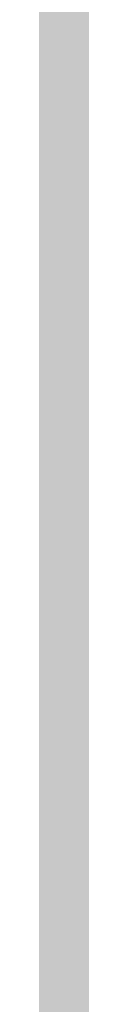
# Model space of a CAD drawing. Units: inches. Extents: x 2083 to 3317, y 1141 to 2115.
# Tile 190 of 256: x 3126.9467 to 3126.9559, y 1263.3548 to 1263.6134. Entities that reach past the tile are written whole.
import ezdxf

# ---------------------------------------------------------------- set-up
doc = ezdxf.new("R2010")
doc.units = ezdxf.units.IN
doc.layers.add('A-ANNO-DIMS', color=2, linetype='Continuous', lineweight=18)
doc.layers.add('A-WALL-PATT', color=251, linetype='Continuous', lineweight=13, true_color=0x636466)
doc.styles.get("Standard").update_dxf_attribs({"font": 'arial.ttf'})
doc.dimstyles.new('ISO-25', dxfattribs={"dimtxt": 12, "dimasz": 12, "dimexe": 1.25, "dimexo": 0.625, "dimtad": 1, "dimlunit": 3, "dimtxsty": 'Standard', "dimcen": 2.5, "dimadec": 0, "dimazin": 0, "dimtfac": 1, "dimtmove": 0, "dimatfit": 3, "dimfxl": 1, "dimarcsym": 0})

# ---------------------------------------------------------------- blocks, each defined once
blk = doc.blocks.new('*D26')
at = {"layer": 'A-ANNO-DIMS', "color": 0, "lineweight": -2, "transparency": 16777216}
for p, q in [((3088.98584, 1274.91509), (3088.98584, 1270.95196)), ((3111.24004, 1274.91509), (3111.24004, 1270.95196)), ((3076.98584, 1272.20196), (2840.26245, 1272.20196)), ((3111.24004, 1272.20196), (3088.98584, 1272.20196)), ((3123.24004, 1272.20196), (3135.24004, 1272.20196))]:
    blk.add_line(p, q, dxfattribs=at)
at = {"layer": 'A-ANNO-DIMS', "color": 0, "transparency": 16777216}
for points in [[(3076.98584, 1274.20196), (3076.98584, 1270.20196), (3088.98584, 1272.20196)], [(3123.24004, 1274.20196), (3123.24004, 1270.20196), (3111.24004, 1272.20196)]]:
    blk.add_solid(points, dxfattribs=at)
at = {"layer": 'Defpoints', "color": 0, "transparency": 16777216}
for p in [(3088.98584, 1275.54009), (3111.24004, 1275.54009), (3088.98584, 1272.20196)]:
    blk.add_point(p, dxfattribs=at)
at = {"layer": 'A-ANNO-DIMS', "color": 0, "transparency": 16777216, "insert": (2952.62415, 1279.0316), "char_height": 12, "attachment_point": 5}
blk.add_mtext('NIGHTSTAND 1\'-10 1/2" TYP.', dxfattribs=at)
blk = doc.blocks.new('*D27')
at = {"layer": 'A-ANNO-DIMS', "color": 0, "lineweight": -2, "transparency": 16777216}
for p, q in [((3114.57817, 1309.79428), (3114.57817, 1321.79428)), ((3111.86504, 1297.79428), (3115.82817, 1297.79428)), ((3114.57817, 1297.79428), (3114.57817, 1275.54009)), ((3111.86504, 1275.54009), (3115.82817, 1275.54009)), ((3114.57817, 1263.54009), (3114.57817, 1140.98859))]:
    blk.add_line(p, q, dxfattribs=at)
at = {"layer": 'A-ANNO-DIMS', "color": 0, "transparency": 16777216}
for points in [[(3112.57817, 1309.79428), (3116.57817, 1309.79428), (3114.57817, 1297.79428)], [(3112.57817, 1263.54009), (3116.57817, 1263.54009), (3114.57817, 1275.54009)]]:
    blk.add_solid(points, dxfattribs=at)
at = {"layer": 'Defpoints', "color": 0, "transparency": 16777216}
for p in [(3111.24004, 1297.79428), (3111.24004, 1275.54009), (3114.57817, 1275.54009)]:
    blk.add_point(p, dxfattribs=at)
at = {"layer": 'A-ANNO-DIMS', "color": 0, "transparency": 16777216, "insert": (3107.74853, 1196.26434), "char_height": 12, "attachment_point": 5, "rotation": 90}
blk.add_mtext('1\'-10 1/2" TYP.', dxfattribs=at)

msp = doc.modelspace()

# ---------------------------------------------------------------- hatches: boundary and pattern name
at = {"layer": 'A-WALL-PATT'}
h = msp.add_hatch(color=256, dxfattribs=at)
h.dxf.hatch_style = 1
h.paths.add_polyline_path([(3126.95978, 2020.76136), (2748.95978, 2020.76136), (2604.95978, 2020.76136), (2226.95978, 2020.76136), (2226.95978, 1702.76136), (2466.95978, 1702.76136), (2466.95978, 1582.76136), (2418.95978, 1582.76136), (2418.95978, 1477.76136), (2226.95978, 1477.76136), (2226.95978, 1263.26136), (2544.95978, 1263.26136), (2544.95978, 1411.76136), (2604.95978, 1411.76136), (2685.95978, 1411.76136), (2685.95978, 1420.76136), (2604.95978, 1420.76136), (2604.95978, 1573.76136), (2604.95978, 1702.76136), (2604.95978, 2011.76136), (2748.95978, 2011.76136), (2748.95978, 1702.76136), (2862.95978, 1702.76136), (2862.95978, 1621.76136), (2871.95978, 1621.76136), (2871.95978, 1702.76136), (2883.95978, 1702.76136), (2883.95978, 1706.93946, -0.026459), (2883.95978, 1711.76136), (2757.95978, 1711.76136), (2757.95978, 1807.76136), (2787.95978, 1807.76136), (2787.95978, 1812.26136), (2757.95978, 1812.26136), (2757.95978, 2011.76136), (2877.95978, 2011.76136), (2877.95978, 1812.26136), (2847.95978, 1812.26136), (2847.95978, 1807.76136), (2889.83574, 1807.76136), (2889.83574, 1812.26136), (2882.45978, 1812.26136), (2882.45978, 2011.76136), (3117.95978, 2011.76136), (3117.95978, 1812.26136), (2937.83574, 1812.26136), (2937.83574, 1807.76136), (2995.70978, 1807.76136), (2995.70978, 1796.11767), (3000.20978, 1796.11767), (3000.20978, 1807.76136), (3117.95978, 1807.76136), (3117.95978, 1711.76136), (3000.20978, 1711.76136), (3000.20978, 1760.11767), (2998.5727, 1760.11767, -0.020711), (2995.70978, 1760.11767), (2995.70978, 1711.76136), (2931.95978, 1711.76136), (2931.95978, 1702.76136), (3126.95978, 1702.76136)])
h.paths.add_polyline_path([(2471.45978, 2011.76136), (2471.45978, 1810.01136), (2462.71694, 1810.01136), (2462.71694, 1805.51136), (2505.95978, 1805.51136), (2505.95978, 1810.01136), (2475.95978, 1810.01136), (2475.95978, 2011.76136), (2595.95978, 2011.76136), (2595.95978, 1810.01136), (2565.95978, 1810.01136), (2565.95978, 1805.51136), (2595.95978, 1805.51136), (2595.95978, 1711.76136), (2235.95978, 1711.76136), (2235.95978, 1805.51136), (2353.70978, 1805.51136), (2353.70978, 1796.05416), (2358.20978, 1796.05416), (2358.20978, 1805.51136), (2414.71694, 1805.51136), (2414.71694, 1810.01136), (2235.95978, 1810.01136), (2235.95978, 2011.76136)], flags=16)
h.paths.add_polyline_path([(2270.20473, 1994.61001), (2270.20473, 1970.61001), (2246.20473, 1970.61001), (2246.20473, 1994.61001)], flags=0)
edge = h.paths.add_edge_path(flags=0)
edge.add_ellipse((2332.02739, 1899.79818), major_axis=(-3.04299, 3.04299), ratio=0.1682525, start_angle=-161.33217, end_angle=-156.30711, ccw=False)
edge.add_ellipse((2333.08204, 1898.74353), major_axis=(-1.05465, 1.05465), ratio=0.4535321, start_angle=-123.37102, end_angle=-94.15911)
edge = h.paths.add_edge_path(flags=0)
edge.add_ellipse((2332.02739, 1968.87629), major_axis=(3.04299, 3.04299), ratio=0.1682525, start_angle=18.66783, end_angle=23.69289)
edge.add_spline(control_points=[(2332.9256, 1970.6911), (2332.22677, 1970.3361), (2330.89371, 1969.65891), (2328.41308, 1970.93214), (2327.20393, 1967.74871), (2324.7096, 1969.95559), (2322.53282, 1967.01235), (2320.01285, 1971.29581), (2317.68031, 1968.15784), (2316.04053, 1967.10205), (2315.4269, 1966.8096)], knot_values=[0, 0, 0, 0, 2.267059, 4.324559, 6.685584, 8.878641, 11.121502, 14.300359, 17.755284, 19.732645, 19.732645, 19.732645, 19.732645], degree=3, periodic=0)
edge.add_ellipse((2332.02739, 1968.87629), major_axis=(3.04299, 3.04299), ratio=0.1682525, start_angle=18.66783, end_angle=23.69289, ccw=False)
edge.add_ellipse((2333.08204, 1969.93094), major_axis=(1.05465, 1.05465), ratio=0.4535321, start_angle=56.62898, end_angle=85.84089, ccw=False)
edge = h.paths.add_edge_path(flags=0)
edge.add_spline(control_points=[(2296.42829, 1967.98791), (2293.6278, 1965.33631), (2287.70362, 1959.72709), (2299.74386, 1949.9957), (2294.53259, 1935.66853), (2290.57323, 1920.60351), (2293.39412, 1909.97369), (2296.18541, 1904.96654)], knot_values=[0.099185, 0.099185, 0.099185, 0.099185, 0.345301, 0.619822, 0.982653, 1.386093, 1.810555, 1.810555, 1.810555, 1.810555], degree=3, periodic=0)
edge.add_spline(control_points=[(2296.18541, 1904.96654), (2297.38358, 1902.6193), (2298.00097, 1901.94931), (2298.55297, 1901.46815)], knot_values=[0.006246, 0.006246, 0.006246, 0.006246, 0.055476, 0.055476, 0.055476, 0.055476], degree=3, periodic=0)
edge.add_spline(control_points=[(2298.55297, 1901.46815), (2297.25861, 1900.92322), (2295.22529, 1900.23213), (2293.06023, 1900.61421), (2292.10142, 1900.78841), (2292.08958, 1900.79057)], knot_values=[0.312835, 0.312835, 0.312835, 0.312835, 0.40178, 0.474987, 0.475903, 0.475903, 0.475903, 0.475903], degree=3, periodic=0)
edge.add_arc((2292.79365, 1904.66411), 3.93701, 215.4209, 259.69818, ccw=False)
edge.add_spline(control_points=[(2289.58531, 1902.3823), (2289.47665, 1902.53509), (2289.36848, 1902.68804), (2289.26086, 1902.84117)], knot_values=[0.102872, 0.102872, 0.102872, 0.102872, 0.116896, 0.116896, 0.116896, 0.116896], degree=3, periodic=0)
edge.add_spline(control_points=[(2289.26086, 1902.84117), (2288.6866, 1902.55019), (2287.64005, 1902.0199), (2285.88134, 1901.87395), (2283.85297, 1901.50435), (2281.71999, 1899.71054), (2278.46699, 1899.49294), (2276.15714, 1901.8832), (2272.25895, 1899.80407), (2267.77761, 1901.84318), (2262.24388, 1900.18403), (2257.41493, 1901.78206), (2254.31837, 1900.72612), (2253.17828, 1900.33734)], knot_values=[0, 0, 0, 0, 1.907977, 3.477176, 5.261074, 7.972851, 11.680248, 13.717921, 16.939592, 22.789562, 27.502503, 33.595215, 37.145618, 37.145618, 37.145618, 37.145618], degree=3, periodic=0)
edge.add_line((2253.17828, 1900.33734), (2250.24424, 1902.84117))
edge.add_line((2250.24424, 1902.84117), (2250.24424, 1965.8333))
edge.add_line((2250.24424, 1965.8333), (2253.17828, 1968.33712))
edge.add_spline(control_points=[(2253.17828, 1968.33712), (2254.31837, 1967.94835), (2257.41493, 1966.89241), (2262.24388, 1968.49043), (2267.77761, 1966.83128), (2271.52673, 1968.53722), (2273.87591, 1967.82829), (2274.2067, 1967.72764)], knot_values=[0, 0, 0, 0, 0.09018, 0.244935, 0.364644, 0.513233, 0.537855, 0.537855, 0.537855, 0.537855], degree=3, periodic=0)
edge.add_arc((2274.35289, 1963.79335), 3.93701, 72.05113, 92.12795, ccw=False)
edge.add_arc((2281.29693, 1985.23), 18.5963, 252.051134, 288.565722)
edge.add_arc((2292.31672, 1956.02888), 12.64608, 71.026788, 113.778218, ccw=False)
edge = h.paths.add_edge_path(flags=0)
edge.add_spline(control_points=[(2274.89941, 1951.85619), (2275.06616, 1951.61659), (2275.23269, 1951.37659), (2275.39799, 1951.13585)], knot_values=[1.409916, 1.409916, 1.409916, 1.409916, 1.43159, 1.43159, 1.43159, 1.43159], degree=3, periodic=0)
edge.add_spline(control_points=[(2275.39799, 1951.13585), (2275.79211, 1950.56189), (2276.17923, 1949.98377), (2276.54555, 1949.3971)], knot_values=[1.358238, 1.358238, 1.358238, 1.358238, 1.409916, 1.409916, 1.409916, 1.409916], degree=3, periodic=0)
edge.add_line((2276.54555, 1949.3971), (2277.43729, 1947.86218))
edge.add_spline(control_points=[(2277.43729, 1947.86218), (2276.30383, 1945.67311), (2274.6397, 1942.42688), (2274.63161, 1938.0939), (2272.79912, 1930.85155), (2274.35643, 1943.89705), (2275.94768, 1947.92336), (2276.54555, 1949.3971)], knot_values=[0.005632, 0.005632, 0.005632, 0.005632, 0.186014, 0.266002, 0.357087, 0.59639, 0.739732, 0.739732, 0.739732, 0.739732], degree=3, periodic=0)
edge.add_spline(control_points=[(2276.54555, 1949.3971), (2276.17923, 1949.98377), (2275.79211, 1950.56189), (2275.39799, 1951.13585)], knot_values=[1.358238, 1.358238, 1.358238, 1.358238, 1.409916, 1.409916, 1.409916, 1.409916], degree=3, periodic=0)
edge.add_spline(control_points=[(2275.39799, 1951.13585), (2274.9425, 1950.08045), (2274.20776, 1948.02527), (2273.9346, 1944.85148), (2272.46853, 1937.62749), (2273.46622, 1945.69647), (2274.70062, 1951.05947), (2274.89941, 1951.85619)], knot_values=[0.104364, 0.104364, 0.104364, 0.104364, 0.189636, 0.269624, 0.36071, 0.600013, 0.644622, 0.644622, 0.644622, 0.644622], degree=3, periodic=0)
h.paths.add_polyline_path([(2269.16751, 1963.12757, -0.357527), (2268.17063, 1960.97637, -0.092561), (2268.17063, 1939.43632, -0.357527), (2269.16751, 1937.28512, -0.357527), (2267.01631, 1938.282, -0.164785), (2254.68558, 1938.282, -0.357527), (2252.53438, 1937.28512, -0.357527), (2253.53126, 1939.43632, -0.092561), (2253.53126, 1960.97637, -0.357527), (2252.53438, 1963.12757, -0.357527), (2254.68558, 1962.13069, -0.164785), (2267.01631, 1962.13069, -0.357527)], flags=0)
h.paths.add_polyline_path([(2248.87407, 1967.8018), (2248.87407, 1957.02771), (2249.45778, 1957.02771), (2249.45778, 1911.64676), (2248.87407, 1911.64676), (2248.87407, 1900.87267), (2246.51186, 1900.87267, 0.197327), (2244.14966, 1902.45687), (2244.14966, 1966.21759, 0.197327), (2246.51186, 1967.8018)], flags=0)
h.paths.add_polyline_path([(2269.16751, 1931.38934, -0.357527), (2268.17063, 1929.23814, -0.092561), (2268.17063, 1907.6981, -0.357527), (2269.16751, 1905.54689, -0.357527), (2267.01631, 1906.54377, -0.164785), (2254.68558, 1906.54377, -0.357527), (2252.53438, 1905.54689, -0.357527), (2253.53126, 1907.6981, -0.092561), (2253.53126, 1929.23814, -0.357527), (2252.53438, 1931.38934, -0.357527), (2254.68558, 1930.39246, -0.164785), (2267.01631, 1930.39246, -0.357527)], flags=0)
edge = h.paths.add_edge_path(flags=0)
edge.add_spline(control_points=[(2276.19686, 1906.7237), (2276.16814, 1909.02893), (2276.11405, 1913.37185), (2270.59842, 1924.92498), (2273.90517, 1919.01278), (2275.92171, 1916.26206), (2275.47457, 1912.40215), (2277.25787, 1910.38062), (2276.69604, 1908.22504), (2276.64622, 1906.81302), (2276.61782, 1906.00841)], knot_values=[0, 0, 0, 0, 8.61026, 16.221274, 18.843057, 23.804898, 27.440828, 29.356102, 31.203478, 33.650687, 33.650687, 33.650687, 33.650687], degree=3, periodic=0)
edge.add_spline(control_points=[(2276.61782, 1906.00841), (2276.62331, 1905.62414), (2276.49774, 1904.62866), (2275.44178, 1903.85473), (2274.93731, 1903.08045), (2274.85908, 1902.84117)], knot_values=[0.156488, 0.156488, 0.156488, 0.156488, 0.184398, 0.231376, 0.250598, 0.250598, 0.250598, 0.250598], degree=3, periodic=0)
edge.add_line((2274.85908, 1902.84117), (2276.50598, 1902.84117))
edge.add_spline(control_points=[(2276.50598, 1902.84117), (2276.78831, 1903.08494), (2277.66507, 1904.1252), (2278.24954, 1904.34074), (2277.65387, 1908.52739), (2278.15567, 1906.22781), (2278.10046, 1905.28595), (2278.84667, 1904.06901), (2277.85679, 1903.41495), (2277.87419, 1902.99105), (2277.90356, 1902.84117)], knot_values=[0.059574, 0.059574, 0.059574, 0.059574, 0.080753, 0.103741, 0.16972, 0.176036, 0.207137, 0.240474, 0.262341, 0.27366, 0.27366, 0.27366, 0.27366], degree=3, periodic=0)
edge.add_line((2277.90356, 1902.84117), (2280.02983, 1902.84117))
edge.add_spline(control_points=[(2280.02983, 1902.84117), (2279.88822, 1903.0884), (2279.49926, 1903.98155), (2280.15228, 1905.93935), (2278.10362, 1909.65776), (2279.76239, 1907.18529), (2280.3279, 1904.87486), (2280.48511, 1903.48959), (2281.46327, 1903.24943), (2281.75834, 1902.9365), (2281.83404, 1902.84117)], knot_values=[0.013856, 0.013856, 0.013856, 0.013856, 0.034874, 0.088867, 0.107879, 0.126738, 0.158714, 0.193757, 0.217487, 0.226722, 0.226722, 0.226722, 0.226722], degree=3, periodic=0)
edge.add_spline(control_points=[(2281.83404, 1902.84117), (2281.78753, 1902.8267), (2281.64702, 1902.78299), (2281.39553, 1902.85949), (2281.08808, 1902.98524), (2280.72068, 1903.0609), (2280.33345, 1903.02573), (2280.12477, 1902.89888), (2280.02983, 1902.84117)], knot_values=[0, 0, 0, 0, 0.14413, 0.435517, 0.749276, 1.153046, 1.548371, 1.878348, 1.878348, 1.878348, 1.878348], degree=3, periodic=0)
edge.add_line((2280.02983, 1902.84117), (2277.90356, 1902.84117))
edge.add_spline(control_points=[(2277.90356, 1902.84117), (2277.89286, 1902.79586), (2277.8654, 1902.67964), (2277.60748, 1902.68748), (2277.27405, 1902.8007), (2276.83792, 1902.61977), (2276.58381, 1902.78926), (2276.50598, 1902.84117)], knot_values=[0, 0, 0, 0, 0.127189, 0.326199, 0.628009, 1.24357, 1.515331, 1.515331, 1.515331, 1.515331], degree=3, periodic=0)
edge.add_line((2276.50598, 1902.84117), (2274.85908, 1902.84117))
edge.add_spline(control_points=[(2274.85908, 1902.84117), (2274.81444, 1902.89859), (2274.72513, 1903.01345), (2274.49348, 1903.11897), (2274.24429, 1902.96054), (2273.93712, 1903.18494), (2273.61404, 1902.98314), (2273.40832, 1902.88304), (2273.32225, 1902.84117)], knot_values=[0, 0, 0, 0, 0.21843, 0.436957, 0.687977, 0.990379, 1.398396, 1.69185, 1.69185, 1.69185, 1.69185], degree=3, periodic=0)
edge.add_spline(control_points=[(2273.32225, 1902.84117), (2273.61674, 1903.44569), (2274.274, 1904.53825), (2276.02724, 1904.5737), (2276.20696, 1906.58364), (2276.19686, 1906.7237)], knot_values=[0.012227, 0.012227, 0.012227, 0.012227, 0.059472, 0.106218, 0.134458, 0.134458, 0.134458, 0.134458], degree=3, periodic=0)
h.paths.add_polyline_path([(2270.77605, 1897.78983), (2270.77605, 1873.78983), (2246.77605, 1873.78983), (2246.77605, 1897.78983)], flags=0)
h.paths.add_polyline_path([(2353.70978, 1760.00506), (2353.70978, 1760.05416), (2358.20978, 1760.05416, -0.033729)], flags=0)
h.paths.add_polyline_path([(2321.81912, 1737.52919), (2341.99533, 1737.52919, -0.414214), (2343.20327, 1736.32124), (2343.20327, 1721.0206, -0.414214), (2341.99533, 1719.81265), (2321.81912, 1719.81265, -0.414214), (2320.61117, 1721.0206), (2320.61117, 1736.32124, -0.414214)], flags=0)
h.paths.add_polyline_path([(2324.23501, 1736.32124), (2339.57944, 1736.32124, -0.414214), (2341.99533, 1733.90535), (2341.99533, 1725.44973, -0.414214), (2339.57944, 1723.03384), (2333.68059, 1723.03384), (2333.84532, 1722.04547, -0.870646), (2335.4254, 1721.82589, -0.767327), (2333.92269, 1721.42324), (2331.29102, 1721.42324, -0.767327), (2329.78832, 1721.82589, -0.870646), (2331.3684, 1722.04547), (2331.53313, 1723.03384), (2324.23501, 1723.03384, -0.414214), (2321.81912, 1725.44973), (2321.81912, 1733.90535, -0.414214)], flags=0)
h.paths.add_polyline_path([(2570.48379, 1928.61544), (2589.68379, 1928.61544), (2590.16883, 1928.61544), (2590.16883, 1904.9934), (2570.48379, 1904.9934)], flags=0)
h.paths.add_polyline_path([(2574.44732, 1927.26382, -1), (2572.82884, 1927.26382, -1)], flags=0)
h.paths.add_polyline_path([(2573.08987, 1926.94088), (2573.92503, 1927.77604), (2574.14774, 1927.55333), (2573.31258, 1926.71817)], flags=0)
h.paths.add_polyline_path([(2578.77906, 1919.72962, -1), (2571.59166, 1919.72962, -1)], flags=0)
h.paths.add_polyline_path([(2578.38536, 1919.72962, -1), (2571.98536, 1919.72962, -1)], flags=0)
h.paths.add_polyline_path([(2331.59576, 1729.47622, -1), (2333.61795, 1729.47622, -1)], flags=0)
h.paths.add_polyline_path([(2578.03423, 1927.26382, -1), (2576.41574, 1927.26382, -1)], flags=0)
h.paths.add_polyline_path([(2576.68885, 1927.53109), (2576.91156, 1927.7538), (2577.74673, 1926.91863), (2577.52402, 1926.69592)], flags=0)
h.paths.add_polyline_path([(2578.13906, 1909.85954, -1), (2572.23166, 1909.85954, -1)], flags=0)
h.paths.add_polyline_path([(2577.74536, 1909.85954, -1), (2572.62536, 1909.85954, -1)], flags=0)
h.paths.add_polyline_path([(2583.79772, 1927.26382, -1), (2582.17923, 1927.26382, -1)], flags=0)
h.paths.add_polyline_path([(2582.71865, 1927.7538), (2583.55381, 1926.91863), (2583.3311, 1926.69592), (2582.49594, 1927.53109)], flags=0)
h.paths.add_polyline_path([(2582.49594, 1927.53109), (2582.71865, 1927.7538), (2583.55381, 1926.91863), (2583.3311, 1926.69592)], flags=0)
h.paths.add_polyline_path([(2587.73906, 1920.52962, -1), (2581.83166, 1920.52962, -1)], flags=0)
h.paths.add_polyline_path([(2587.34536, 1920.52962, -1), (2582.22536, 1920.52962, -1)], flags=0)
h.paths.add_polyline_path([(2587.38462, 1927.26382, -1), (2585.76613, 1927.26382, -1)], flags=0)
h.paths.add_polyline_path([(2586.08199, 1926.98025), (2586.91716, 1927.81541), (2587.13987, 1927.5927), (2586.3047, 1926.75754)], flags=0)
h.paths.add_polyline_path([(2588.37906, 1910.65954, -1), (2581.19166, 1910.65954, -1)], flags=0)
h.paths.add_polyline_path([(2587.98536, 1910.65954, -1), (2581.58536, 1910.65954, -1)], flags=0)
h.paths.add_polyline_path([(2417.16773, 1729.4779), (2437.34394, 1729.4779, -0.414214), (2438.55188, 1728.26995), (2438.55188, 1712.96931, -0.414214), (2437.34394, 1711.76136), (2417.16773, 1711.76136, -0.414214), (2415.95978, 1712.96931), (2415.95978, 1728.26995, -0.414214)], flags=0)
h.paths.add_polyline_path([(2419.58362, 1728.26995), (2434.92805, 1728.26995, -0.414214), (2437.34394, 1725.85406), (2437.34394, 1717.39844, -0.414214), (2434.92805, 1714.98255), (2429.0292, 1714.98255), (2429.19393, 1713.99418, -0.870646), (2430.77401, 1713.7746, -0.767327), (2429.2713, 1713.37195), (2426.63963, 1713.37195, -0.767327), (2425.13693, 1713.7746, -0.870646), (2426.71701, 1713.99418), (2426.88174, 1714.98255), (2419.58362, 1714.98255, -0.414214), (2417.16773, 1717.39844), (2417.16773, 1725.85406, -0.414214)], flags=0)
h.paths.add_polyline_path([(2419.58362, 1728.26995), (2434.92805, 1728.26995, -0.414214), (2437.34394, 1725.85406), (2437.34394, 1717.39844, -0.414214), (2434.92805, 1714.98255), (2429.0292, 1714.98255), (2428.35812, 1719.00903), (2427.55282, 1719.00903), (2426.88174, 1714.98255), (2419.58362, 1714.98255, -0.414214), (2417.16773, 1717.39844), (2417.16773, 1725.85406, -0.414214)], flags=0)
h.paths.add_polyline_path([(2426.94437, 1721.42492, -1), (2428.96656, 1721.42492, -1)], flags=0)
h.paths.add_polyline_path([(2475.95978, 1702.76136), (2595.95978, 1702.76136), (2595.95978, 1582.76136), (2475.95978, 1582.76136)], flags=16)
h.paths.add_polyline_path([(2427.95978, 1573.76136), (2595.95978, 1573.76136), (2595.95978, 1468.76136), (2595.95978, 1420.76136), (2384.45978, 1420.76136), (2384.45978, 1468.76136), (2427.95978, 1468.76136)], flags=16)
h.paths.add_polyline_path([(2379.95978, 1468.76136), (2379.95978, 1420.76136), (2235.95978, 1420.76136), (2235.95978, 1468.76136)], flags=16)
h.paths.add_polyline_path([(2317.816, 1466.69577), (2337.9922, 1466.69577, -0.414214), (2339.20015, 1465.48782), (2339.20015, 1450.18718, -0.414214), (2337.9922, 1448.97923), (2317.816, 1448.97923, -0.414214), (2316.60805, 1450.18718), (2316.60805, 1465.48782, -0.414214)], flags=0)
h.paths.add_polyline_path([(2320.23189, 1465.48782), (2335.57631, 1465.48782, -0.414214), (2337.9922, 1463.07193), (2337.9922, 1454.61631, -0.414214), (2335.57631, 1452.20042), (2329.67747, 1452.20042), (2329.84219, 1451.21205, -0.870646), (2331.42228, 1450.99247, -0.767327), (2329.91957, 1450.58983), (2327.2879, 1450.58983, -0.767327), (2325.7852, 1450.99247, -0.870646), (2327.36528, 1451.21205), (2327.53001, 1452.20042), (2320.23189, 1452.20042, -0.414214), (2317.816, 1454.61631), (2317.816, 1463.07193, -0.414214)], flags=0)
h.paths.add_polyline_path([(2320.23189, 1465.48782), (2335.57631, 1465.48782, -0.414214), (2337.9922, 1463.07193), (2337.9922, 1454.61631, -0.414214), (2335.57631, 1452.20042), (2329.67747, 1452.20042), (2329.00638, 1456.22691), (2328.20109, 1456.22691), (2327.53001, 1452.20042), (2320.23189, 1452.20042, -0.414214), (2317.816, 1454.61631), (2317.816, 1463.07193, -0.414214)], flags=0)
h.paths.add_polyline_path([(2327.59264, 1458.6428, -1), (2329.61483, 1458.6428, -1)], flags=0)
h.paths.add_polyline_path([(2244.41174, 1433.34045), (2241.92094, 1433.34045, -0.414214), (2240.01786, 1435.24354), (2240.01786, 1440.95281, -0.414211), (2241.92093, 1442.8559), (2244.41174, 1442.8559, -1.976472)], flags=0)
h.paths.add_polyline_path([(2245.35689, 1434.39754, -0.414214), (2245.35689, 1441.79881, -2.144098)], flags=0)
h.paths.add_polyline_path([(2535.95978, 1416.26136), (2535.95978, 1272.26136), (2235.95978, 1272.26136), (2235.95978, 1416.26136)], flags=16)
h.paths.add_polyline_path([(2260.11956, 1384.29284), (2260.11956, 1362.03865), (2237.86537, 1362.03865), (2237.86537, 1384.29284)], flags=0)
edge = h.paths.add_edge_path(flags=0)
edge.add_line((2318.25185, 1362.0933), (2318.1458, 1362.00097))
edge.add_ellipse((2317.44512, 1360.43104), major_axis=(2.82164, 2.82164), ratio=0.1682525, start_angle=18.66783, end_angle=20.94813, ccw=False)
edge.add_ellipse((2318.42305, 1361.40897), major_axis=(0.97793, 0.97793), ratio=0.4535321, start_angle=56.62898, end_angle=70.2262, ccw=False)
edge = h.paths.add_edge_path(flags=0)
edge.add_line((2319.10737, 1295.57108), (2319.01504, 1295.67713))
edge.add_ellipse((2317.44512, 1296.37781), major_axis=(-2.82164, 2.82164), ratio=0.1682525, start_angle=-161.33217, end_angle=-159.05187, ccw=False)
edge.add_ellipse((2318.42305, 1295.39988), major_axis=(-0.97793, 0.97793), ratio=0.4535321, start_angle=-123.37102, end_angle=-109.7738)
edge = h.paths.add_edge_path(flags=0)
edge.add_spline(control_points=[(2284.21035, 1301.17022), (2284.58069, 1300.44472), (2284.89119, 1299.89202), (2285.15955, 1299.46102)], knot_values=[0.039066, 0.039066, 0.039066, 0.039066, 0.055476, 0.055476, 0.055476, 0.055476], degree=3, periodic=0)
edge.add_line((2285.15955, 1299.46102), (2284.21035, 1301.17022))
edge = h.paths.add_edge_path(flags=0)
edge.add_line((2280.41246, 1297.29801), (2283.36999, 1297.03612))
edge.add_line((2283.36999, 1297.03612), (2286.40569, 1297.92631))
edge.add_spline(control_points=[(2286.40569, 1297.92631), (2285.30549, 1297.46312), (2284.34478, 1297.12915), (2283.36999, 1297.03612)], knot_values=[0.394369, 0.394369, 0.394369, 0.394369, 0.475903, 0.475903, 0.475903, 0.475903], degree=3, periodic=0)
edge.add_spline(control_points=[(2283.36999, 1297.03612), (2283.28139, 1297.02767), (2282.31629, 1296.95734), (2281.3125, 1297.13448), (2280.42344, 1297.29602), (2280.41246, 1297.29801)], knot_values=[0.312835, 0.312835, 0.312835, 0.312835, 0.320246, 0.393453, 0.394369, 0.394369, 0.394369, 0.394369], degree=3, periodic=0)
edge = h.paths.add_edge_path(flags=0)
edge.add_line((2284.43556, 1359.60729), (2280.44629, 1355.32805))
edge.add_line((2280.44629, 1355.32805), (2279.57999, 1351.01775))
edge.add_line((2279.57999, 1351.01775), (2282.41297, 1346.58043))
edge.add_spline(control_points=[(2282.41297, 1346.58043), (2283.15333, 1345.58924), (2284.2529, 1344.0289), (2284.80104, 1342.38717), (2284.93516, 1341.80554)], knot_values=[1.240098, 1.240098, 1.240098, 1.240098, 1.332892, 1.382712, 1.382712, 1.382712, 1.382712], degree=3, periodic=0)
edge.add_spline(control_points=[(2284.93516, 1341.80554), (2285.31911, 1340.1406), (2285.23303, 1338.4092), (2284.90994, 1336.65412)], knot_values=[1.097484, 1.097484, 1.097484, 1.097484, 1.240098, 1.240098, 1.240098, 1.240098], degree=3, periodic=0)
edge.add_spline(control_points=[(2284.90994, 1336.65412), (2284.58685, 1334.89904), (2284.02675, 1333.12027), (2283.46264, 1331.36058)], knot_values=[0.95487, 0.95487, 0.95487, 0.95487, 1.097484, 1.097484, 1.097484, 1.097484], degree=3, periodic=0)
edge.add_line((2283.46264, 1331.36058), (2281.89038, 1326.15336))
edge.add_line((2281.89038, 1326.15336), (2280.75626, 1321.05609))
edge.add_line((2280.75626, 1321.05609), (2280.2992, 1316.00198))
edge.add_line((2280.2992, 1316.00198), (2280.71593, 1310.95007))
edge.add_line((2280.71593, 1310.95007), (2282.02809, 1305.97214))
edge.add_line((2282.02809, 1305.97214), (2284.21035, 1301.17022))
edge.add_spline(control_points=[(2284.21035, 1301.17022), (2283.34073, 1302.73019), (2282.6119, 1304.33649), (2282.02809, 1305.97214)], knot_values=[0.099185, 0.099185, 0.099185, 0.099185, 0.241799, 0.241799, 0.241799, 0.241799], degree=3, periodic=0)
edge.add_spline(control_points=[(2282.02809, 1305.97214), (2281.44428, 1307.60778), (2281.00549, 1309.27276), (2280.71593, 1310.95007)], knot_values=[0.241799, 0.241799, 0.241799, 0.241799, 0.384413, 0.384413, 0.384413, 0.384413], degree=3, periodic=0)
edge.add_spline(control_points=[(2280.71593, 1310.95007), (2280.43324, 1312.58761), (2280.28939, 1314.27696), (2280.29889, 1315.96203), (2280.2992, 1316.00198)], knot_values=[0.384413, 0.384413, 0.384413, 0.384413, 0.523647, 0.527028, 0.527028, 0.527028, 0.527028], degree=3, periodic=0)
edge.add_spline(control_points=[(2280.2992, 1316.00198), (2280.31233, 1317.68696), (2280.47787, 1319.36793), (2280.75626, 1321.05609)], knot_values=[0.527028, 0.527028, 0.527028, 0.527028, 0.669642, 0.669642, 0.669642, 0.669642], degree=3, periodic=0)
edge.add_spline(control_points=[(2280.75626, 1321.05609), (2281.03465, 1322.74425), (2281.42588, 1324.43961), (2281.89038, 1326.15336)], knot_values=[0.669642, 0.669642, 0.669642, 0.669642, 0.812256, 0.812256, 0.812256, 0.812256], degree=3, periodic=0)
edge.add_spline(control_points=[(2281.89038, 1326.15336), (2282.26438, 1327.53325), (2282.78787, 1329.26181), (2283.35275, 1331.01778), (2283.46264, 1331.36058)], knot_values=[0.812256, 0.812256, 0.812256, 0.812256, 0.927087, 0.95487, 0.95487, 0.95487, 0.95487], degree=3, periodic=0)
edge.add_line((2283.46264, 1331.36058), (2284.90994, 1336.65412))
edge.add_line((2284.90994, 1336.65412), (2284.93516, 1341.80554))
edge.add_line((2284.93516, 1341.80554), (2282.41297, 1346.58043))
edge.add_spline(control_points=[(2282.41297, 1346.58043), (2281.27513, 1348.10379), (2280.07845, 1349.57032), (2279.57999, 1351.01775)], knot_values=[1.382712, 1.382712, 1.382712, 1.382712, 1.525326, 1.525326, 1.525326, 1.525326], degree=3, periodic=0)
edge.add_spline(control_points=[(2279.57999, 1351.01775), (2279.44328, 1351.41472), (2279.13631, 1352.85692), (2279.73519, 1354.29039), (2280.44629, 1355.32805)], knot_values=[1.525326, 1.525326, 1.525326, 1.525326, 1.564439, 1.667941, 1.667941, 1.667941, 1.667941], degree=3, periodic=0)
edge.add_spline(control_points=[(2280.44629, 1355.32805), (2281.42611, 1356.75784), (2282.93084, 1358.18256), (2284.43556, 1359.60729)], knot_values=[1.667941, 1.667941, 1.667941, 1.667941, 1.810555, 1.810555, 1.810555, 1.810555], degree=3, periodic=0)
edge.add_arc((2280.62307, 1348.51818), 11.72618, 71.026788, 113.778218)
edge.add_arc((2270.40489, 1375.59516), 17.24357, 252.051134, 288.565722, ccw=False)
edge.add_arc((2263.96597, 1355.71785), 3.65062, 72.05113, 92.12795)
edge.add_arc((2263.96597, 1355.71785), 3.65062, 92.12795, 177.98513)
edge.add_spline(control_points=[(2260.3176, 1355.8462), (2260.26042, 1354.22067), (2260.55128, 1350.18655), (2262.99934, 1346.76625), (2264.47274, 1344.64902)], knot_values=[1.43159, 1.43159, 1.43159, 1.43159, 1.564144, 1.770695, 1.770695, 1.770695, 1.770695], degree=3, periodic=0)
edge.add_line((2264.47274, 1344.64902), (2264.93559, 1343.98253))
edge.add_spline(control_points=[(2263.80104, 1340.24811), (2263.84324, 1340.51409), (2264.06724, 1341.75647), (2264.51269, 1343.00245), (2264.93505, 1343.98108)], knot_values=[0.53657, 0.53657, 0.53657, 0.53657, 0.559349, 0.644622, 0.644622, 0.644622, 0.644622], degree=3, periodic=0)
edge.add_spline(control_points=[(2264.93505, 1343.98108), (2265.11777, 1343.71497), (2265.29888, 1343.44791), (2265.47676, 1343.17936)], knot_values=[1.384077, 1.384077, 1.384077, 1.384077, 1.409916, 1.409916, 1.409916, 1.409916], degree=3, periodic=0)
edge.add_spline(control_points=[(2265.47676, 1343.17936), (2265.65464, 1342.91082), (2265.8293, 1342.64081), (2265.99913, 1342.36881)], knot_values=[1.358238, 1.358238, 1.358238, 1.358238, 1.384077, 1.384077, 1.384077, 1.384077], degree=3, periodic=0)
edge.add_line((2265.99913, 1342.36881), (2266.82601, 1340.94555))
edge.add_spline(control_points=[(2266.82601, 1340.94555), (2268.8944, 1337.08969), (2271.39817, 1325.843), (2270.51616, 1310.56856), (2275.91938, 1301.86061), (2277.78951, 1299.19945)], knot_values=[0.116896, 0.116896, 0.116896, 0.116896, 0.472987, 1.050969, 1.313793, 1.313793, 1.313793, 1.313793], degree=3, periodic=0)
edge.add_spline(control_points=[(2277.78951, 1299.19945), (2277.83941, 1299.12845), (2277.88943, 1299.0575), (2277.93957, 1298.98658)], knot_values=[0.109884, 0.109884, 0.109884, 0.109884, 0.116896, 0.116896, 0.116896, 0.116896], degree=3, periodic=0)
edge.add_line((2277.93957, 1298.98658), (2277.78885, 1299.19911))
edge.add_spline(control_points=[(2277.78885, 1299.19911), (2277.25658, 1298.92941), (2276.28635, 1298.4379), (2275.03935, 1298.33442), (2274.38333, 1298.2389), (2274.21525, 1298.20934)], knot_values=[33.12187, 33.12187, 33.12187, 33.12187, 35.029056, 36.598255, 37.144827, 37.144827, 37.144827, 37.144827], degree=3, periodic=0)
edge.add_line((2274.21525, 1298.20934), (2273.07315, 1297.89296))
edge.add_spline(control_points=[(2273.07315, 1297.89296), (2272.32294, 1297.57978), (2271.03915, 1296.51051), (2269.24839, 1296.22606), (2268.4231, 1296.37465)], knot_values=[26.532584, 26.532584, 26.532584, 26.532584, 29.198919, 31.839101, 31.839101, 31.839101, 31.839101], degree=3, periodic=0)
edge.add_line((2268.4231, 1296.37465), (2263.8785, 1297.45753))
edge.add_spline(control_points=[(2263.8785, 1297.45753), (2263.55608, 1297.35943), (2261.86031, 1296.83869), (2260.23878, 1297.28241), (2258.93345, 1297.51646)], knot_values=[15.919551, 15.919551, 15.919551, 15.919551, 16.939592, 21.226067, 21.226067, 21.226067, 21.226067], degree=3, periodic=0)
edge.add_line((2258.93345, 1297.51646), (2254.05523, 1297.32901))
edge.add_spline(control_points=[(2254.05523, 1297.32901), (2253.75553, 1297.29582), (2252.11368, 1297.16517), (2250.46187, 1297.54422), (2249.12969, 1297.66788)], knot_values=[5.306517, 5.306517, 5.306517, 5.306517, 6.276435, 10.613034, 10.613034, 10.613034, 10.613034], degree=3, periodic=0)
edge.add_line((2249.12969, 1297.66788), (2244.33165, 1296.87776))
edge.add_line((2244.33165, 1296.87776), (2241.61103, 1299.19945))
edge.add_line((2241.61103, 1299.19945), (2241.61103, 1357.6094))
edge.add_line((2241.61103, 1357.6094), (2244.33165, 1359.9311))
edge.add_line((2244.33165, 1359.9311), (2252.72882, 1359.54269))
edge.add_spline(control_points=[(2252.72882, 1359.54269), (2252.87094, 1359.54644), (2253.30574, 1359.54817), (2253.73984, 1359.51427), (2254.03174, 1359.48243)], knot_values=[0.233291, 0.233291, 0.233291, 0.233291, 0.244935, 0.268927, 0.268927, 0.268927, 0.268927], degree=3, periodic=0)
edge.add_line((2254.03174, 1359.48243), (2259.58719, 1359.41639))
edge.add_spline(control_points=[(2259.58719, 1359.41639), (2260.67707, 1359.6285), (2262.0732, 1359.897), (2263.52369, 1359.45928), (2263.83042, 1359.36595)], knot_values=[0.422516, 0.422516, 0.422516, 0.422516, 0.513233, 0.537855, 0.537855, 0.537855, 0.537855], degree=3, periodic=0)
edge.add_arc((2263.96597, 1355.71785), 3.65062, 72.05113, 92.12795, ccw=False)
edge.add_arc((2270.40489, 1375.59516), 17.24357, 252.051134, 288.565722)
edge.add_arc((2280.62307, 1348.51818), 11.72618, 71.026788, 113.778218, ccw=False)
h.paths.add_polyline_path([(2240.34053, 1359.43471), (2240.34053, 1349.44435), (2240.88178, 1349.44435), (2240.88178, 1307.3645), (2240.34053, 1307.3645), (2240.34053, 1297.37414), (2238.15016, 1297.37414, 0.197327), (2235.95978, 1298.84311), (2235.95978, 1357.96575, 0.197327), (2238.15016, 1359.43471)], flags=0)
h.paths.add_polyline_path([(2259.15779, 1355.1005, -0.357527), (2258.23342, 1353.10578, -0.092561), (2258.23342, 1333.1326, -0.357527), (2259.15779, 1331.13788, -0.357527), (2257.16307, 1332.06225, -0.164785), (2245.7293, 1332.06225, -0.357527), (2243.73458, 1331.13788, -0.357527), (2244.65895, 1333.1326, -0.092561), (2244.65895, 1353.10578, -0.357527), (2243.73458, 1355.1005, -0.357527), (2245.7293, 1354.17613, -0.164785), (2257.16307, 1354.17613, -0.357527)], flags=0)
edge = h.paths.add_edge_path(flags=0)
edge.add_line((2265.99913, 1342.36881), (2266.82601, 1340.94555))
edge.add_line((2266.82601, 1340.94555), (2265.30756, 1337.81407))
edge.add_line((2265.30756, 1337.81407), (2264.35823, 1334.65294))
edge.add_line((2264.35823, 1334.65294), (2264.26201, 1333.7997))
edge.add_spline(control_points=[(2264.26201, 1333.7997), (2264.20836, 1333.18705), (2264.16206, 1332.36553), (2264.00714, 1331.41393), (2263.96905, 1331.20183)], knot_values=[0.464444, 0.464444, 0.464444, 0.464444, 0.516691, 0.531608, 0.531608, 0.531608, 0.531608], degree=3, periodic=0)
edge.add_spline(control_points=[(2263.96905, 1331.20183), (2263.77453, 1330.11887), (2263.42437, 1328.79084), (2263.25742, 1328.53065), (2263.23403, 1328.51461)], knot_values=[0.372682, 0.372682, 0.372682, 0.372682, 0.44885, 0.464444, 0.464444, 0.464444, 0.464444], degree=3, periodic=0)
edge.add_spline(control_points=[(2263.23403, 1328.51461), (2263.09638, 1328.42023), (2263.13117, 1329.30148), (2263.27495, 1330.61575)], knot_values=[0.280919, 0.280919, 0.280919, 0.280919, 0.372682, 0.372682, 0.372682, 0.372682], degree=3, periodic=0)
edge.add_spline(control_points=[(2263.27495, 1330.61575), (2263.41874, 1331.93002), (2263.67152, 1333.67732), (2263.96985, 1335.31503)], knot_values=[0.189157, 0.189157, 0.189157, 0.189157, 0.280919, 0.280919, 0.280919, 0.280919], degree=3, periodic=0)
edge.add_spline(control_points=[(2263.96985, 1335.31503), (2264.1005, 1336.03219), (2264.41878, 1337.62191), (2264.75485, 1338.86443), (2264.94742, 1339.49112)], knot_values=[0.097394, 0.097394, 0.097394, 0.097394, 0.137578, 0.189157, 0.189157, 0.189157, 0.189157], degree=3, periodic=0)
edge.add_spline(control_points=[(2264.94742, 1339.49112), (2265.29002, 1340.60605), (2265.64424, 1341.494), (2265.99913, 1342.36881)], knot_values=[0.005632, 0.005632, 0.005632, 0.005632, 0.097394, 0.097394, 0.097394, 0.097394], degree=3, periodic=0)
h.paths.add_polyline_path([(2259.15779, 1325.67097, -0.357527), (2258.23342, 1323.67625, -0.092561), (2258.23342, 1303.70307, -0.357527), (2259.15779, 1301.70835, -0.357527), (2257.16307, 1302.63272, -0.164785), (2245.7293, 1302.63272, -0.357527), (2243.73458, 1301.70835, -0.357527), (2244.65895, 1303.70307, -0.092561), (2244.65895, 1323.67625, -0.357527), (2243.73458, 1325.67097, -0.357527), (2245.7293, 1324.74661, -0.164785), (2257.16307, 1324.74661, -0.357527)], flags=0)
edge = h.paths.add_edge_path(flags=0)
edge.add_spline(control_points=[(2261.70894, 1317.31142), (2261.67948, 1317.41758), (2261.76186, 1317.38853), (2262.49074, 1316.08987), (2262.96218, 1315.3009)], knot_values=[14.955861, 14.955861, 14.955861, 14.955861, 16.221274, 18.694826, 18.694826, 18.694826, 18.694826], degree=3, periodic=0)
edge.add_spline(control_points=[(2262.96218, 1315.3009), (2262.99044, 1315.25362), (2263.7021, 1314.06738), (2264.34898, 1313.12715), (2264.73005, 1312.16415)], knot_values=[18.694826, 18.694826, 18.694826, 18.694826, 18.843057, 22.433791, 22.433791, 22.433791, 22.433791], degree=3, periodic=0)
edge.add_spline(control_points=[(2264.73005, 1312.16415), (2264.87556, 1311.79644), (2265.17687, 1310.76981), (2265.14307, 1309.55926), (2265.24774, 1308.82419)], knot_values=[22.433791, 22.433791, 22.433791, 22.433791, 23.804898, 26.172756, 26.172756, 26.172756, 26.172756], degree=3, periodic=0)
edge.add_line((2265.24774, 1308.82419), (2265.85077, 1307.17189))
edge.add_spline(control_points=[(2265.85077, 1307.17189), (2266.06502, 1306.82168), (2266.38439, 1306.33225), (2266.4244, 1305.78055), (2266.42037, 1305.61122)], knot_values=[28.062562, 28.062562, 28.062562, 28.062562, 29.356102, 29.911721, 29.911721, 29.911721, 29.911721], degree=3, periodic=0)
edge.add_spline(control_points=[(2266.42037, 1305.61122), (2266.41612, 1305.43259), (2266.394, 1305.25), (2266.36478, 1305.06586)], knot_values=[29.911721, 29.911721, 29.911721, 29.911721, 30.497837, 30.497837, 30.497837, 30.497837], degree=3, periodic=0)
edge.add_line((2266.36478, 1305.06586), (2266.06615, 1302.1363))
edge.add_spline(control_points=[(2266.06615, 1302.1363), (2266.07124, 1301.77998), (2265.99808, 1301.19998), (2265.66327, 1300.75896), (2265.50891, 1300.58588)], knot_values=[0.156488, 0.156488, 0.156488, 0.156488, 0.184398, 0.203543, 0.203543, 0.203543, 0.203543], degree=3, periodic=0)
edge.add_line((2265.50891, 1300.58588), (2264.43534, 1299.19945))
edge.add_line((2264.43534, 1299.19945), (2265.96244, 1299.19945))
edge.add_line((2265.96244, 1299.19945), (2267.33599, 1301.17528))
edge.add_line((2267.33599, 1301.17528), (2267.31167, 1301.98624))
edge.add_spline(control_points=[(2267.31167, 1301.98624), (2267.26111, 1302.8624), (2267.16021, 1303.73713), (2267.27149, 1303.3259)], knot_values=[0.126229, 0.126229, 0.126229, 0.126229, 0.166617, 0.166617, 0.166617, 0.166617], degree=3, periodic=0)
edge.add_spline(control_points=[(2267.27149, 1303.3259), (2267.28003, 1303.2943), (2267.30979, 1303.17537), (2267.37345, 1302.88361), (2267.40612, 1302.68283), (2267.41793, 1302.60103)], knot_values=[0.166617, 0.166617, 0.166617, 0.166617, 0.16972, 0.176036, 0.180765, 0.180765, 0.180765, 0.180765], degree=3, periodic=0)
edge.add_spline(control_points=[(2267.74389, 1300.9875), (2267.68758, 1301.15094), (2267.48052, 1301.65666), (2267.48375, 1302.14479), (2267.41793, 1302.60103)], knot_values=[0.180765, 0.180765, 0.180765, 0.180765, 0.193767, 0.220139, 0.220139, 0.220139, 0.220139], degree=3, periodic=0)
edge.add_line((2267.41793, 1302.60103), (2267.74389, 1300.9875))
edge.add_spline(control_points=[(2267.74389, 1300.9875), (2267.83196, 1300.73188), (2267.93202, 1300.3099), (2267.55484, 1299.97452), (2267.42937, 1299.82921)], knot_values=[0.220139, 0.220139, 0.220139, 0.220139, 0.240474, 0.25489, 0.25489, 0.25489, 0.25489], degree=3, periodic=0)
edge.add_line((2267.42937, 1299.82921), (2267.25836, 1299.19945))
edge.add_line((2267.25836, 1299.19945), (2269.22996, 1299.19945))
edge.add_spline(control_points=[(2269.22996, 1299.19945), (2269.09865, 1299.42869), (2268.84277, 1300.01625), (2269.01157, 1300.91592), (2268.9468, 1301.66074)], knot_values=[0.013856, 0.013856, 0.013856, 0.013856, 0.034874, 0.067073, 0.067073, 0.067073, 0.067073], degree=3, periodic=0)
edge.add_line((2268.9468, 1301.66074), (2268.43158, 1303.60311))
edge.add_spline(control_points=[(2268.43158, 1303.60311), (2268.1756, 1304.19237), (2267.59621, 1305.2513), (2268.0407, 1304.62321), (2268.25139, 1304.28242)], knot_values=[0.090155, 0.090155, 0.090155, 0.090155, 0.107879, 0.120289, 0.120289, 0.120289, 0.120289], degree=3, periodic=0)
edge.add_spline(control_points=[(2268.25139, 1304.28242), (2268.36088, 1304.10533), (2269.05775, 1302.91798), (2269.38269, 1301.59042), (2269.52141, 1300.77593), (2269.57522, 1300.55578)], knot_values=[0.120289, 0.120289, 0.120289, 0.120289, 0.126738, 0.158714, 0.173506, 0.173506, 0.173506, 0.173506], degree=3, periodic=0)
edge.add_line((2269.57522, 1300.55578), (2270.6858, 1299.42126))
edge.add_spline(control_points=[(2270.6858, 1299.42126), (2270.76722, 1299.35725), (2270.83785, 1299.2814), (2270.90292, 1299.19945)], knot_values=[0.21816, 0.21816, 0.21816, 0.21816, 0.226722, 0.226722, 0.226722, 0.226722], degree=3, periodic=0)
edge.add_line((2270.9372, 1299.19291), (2270.90292, 1299.19945))
edge.add_spline(control_points=[(2270.90292, 1299.19945), (2270.85981, 1299.18603), (2270.72951, 1299.1455), (2270.49631, 1299.21644), (2270.27166, 1299.30832), (2270.12102, 1299.34796), (2270.06334, 1299.35956)], knot_values=[0.939174, 0.939174, 0.939174, 0.939174, 1.083304, 1.374691, 1.68845, 1.878348, 1.878348, 1.878348, 1.878348], degree=3, periodic=0)
edge.add_line((2270.06334, 1299.35956), (2269.22996, 1299.19945))
edge.add_line((2269.22996, 1299.19945), (2267.25836, 1299.19945))
edge.add_spline(control_points=[(2267.25836, 1299.19945), (2267.24843, 1299.15743), (2267.22297, 1299.04967), (2266.98382, 1299.05694), (2266.80921, 1299.11623), (2266.6769, 1299.10909), (2266.63653, 1299.10481)], knot_values=[0.757665, 0.757665, 0.757665, 0.757665, 0.884854, 1.083864, 1.385675, 1.515331, 1.515331, 1.515331, 1.515331], degree=3, periodic=0)
edge.add_spline(control_points=[(2266.63653, 1299.10481), (2266.48522, 1299.08879), (2266.23581, 1299.01712), (2266.03461, 1299.15132), (2265.96244, 1299.19945)], knot_values=[0, 0, 0, 0, 0.485905, 0.757665, 0.757665, 0.757665, 0.757665], degree=3, periodic=0)
edge.add_line((2265.96244, 1299.19945), (2264.43534, 1299.19945))
edge.add_line((2264.43534, 1299.19945), (2263.85844, 1299.36712))
edge.add_spline(control_points=[(2263.85844, 1299.36712), (2263.81894, 1299.37091), (2263.77953, 1299.38572), (2263.74013, 1299.4015)], knot_values=[0.845925, 0.845925, 0.845925, 0.845925, 0.978627, 0.978627, 0.978627, 0.978627], degree=3, periodic=0)
edge.add_line((2263.72179, 1299.39643), (2263.01031, 1299.19945))
edge.add_spline(control_points=[(2263.01031, 1299.19945), (2263.24579, 1299.68286), (2263.50603, 1300.12811), (2263.87349, 1300.40803)], knot_values=[0.012227, 0.012227, 0.012227, 0.012227, 0.052971, 0.052971, 0.052971, 0.052971], degree=3, periodic=0)
edge.add_spline(control_points=[(2263.87349, 1300.40803), (2263.93213, 1300.4527), (2264.08424, 1300.55298), (2264.25519, 1300.62422), (2264.35969, 1300.66475)], knot_values=[0.052971, 0.052971, 0.052971, 0.052971, 0.059472, 0.069086, 0.069086, 0.069086, 0.069086], degree=3, periodic=0)
edge.add_line((2264.35969, 1300.66475), (2265.1419, 1301.07777))
edge.add_line((2265.1419, 1301.07777), (2265.67581, 1302.79956))
edge.add_line((2265.67581, 1302.79956), (2265.5407, 1305.70407))
edge.add_line((2265.5407, 1305.70407), (2264.80307, 1309.32772))
edge.add_line((2264.80307, 1309.32772), (2263.04053, 1314.09179))
edge.add_spline(control_points=[(2263.04053, 1314.09179), (2262.38357, 1315.67144), (2261.79597, 1316.99775), (2261.70894, 1317.31142)], knot_values=[11.216896, 11.216896, 11.216896, 11.216896, 14.955861, 14.955861, 14.955861, 14.955861], degree=3, periodic=0)
h.paths.add_polyline_path([(2871.95978, 1416.26136), (2895.91005, 1416.26136), (2895.91005, 1420.76136), (2871.95978, 1420.76136), (2871.95978, 1501.76136), (2862.95978, 1501.76136), (2862.95978, 1420.76136), (2805.95978, 1420.76136), (2805.95978, 1411.76136), (2862.95978, 1411.76136), (2862.95978, 1263.26136), (3126.95978, 1263.26136), (3126.95978, 1411.76136), (3126.95978, 1486.76136), (2943.95978, 1486.76136), (2943.95978, 1477.76136), (2967.86031, 1477.76136), (2967.86031, 1420.76136), (2943.91005, 1420.76136), (2943.91005, 1416.26136), (3117.95978, 1416.26136), (3117.95978, 1420.76136), (2972.36031, 1420.76136), (2972.36031, 1477.76136), (3117.95978, 1477.76136), (3117.95978, 1420.76136), (3117.95978, 1272.26136), (2871.95978, 1272.26136)], flags=0)
h.paths.add_polyline_path([(2457.12563, 1485.94251), (2527.60265, 1485.94251), (2527.60265, 1537.6357), (2457.12563, 1537.6357)], flags=8)
h.paths.add_polyline_path([(2481.00506, 1609.9818), (2590.76582, 1609.9818), (2590.76582, 1682.00336), (2481.00506, 1682.00336)], flags=8)
h.paths.add_polyline_path([(2483.08502, 1729.12678), (2553.56205, 1729.12678), (2553.56205, 1780.81998), (2483.08502, 1780.81998)], flags=8)
h = msp.add_hatch(color=256, dxfattribs=at)
h.dxf.hatch_style = 1
h.paths.add_polyline_path([(3126.95978, 1486.76136), (2943.95978, 1486.76136), (2943.95978, 1477.76136), (2967.86031, 1477.76136), (2967.86031, 1420.76136), (2943.91005, 1420.76136), (2943.91005, 1416.26136), (3117.95978, 1416.26136), (3117.95978, 1420.76136), (2972.36031, 1420.76136), (2972.36031, 1477.76136), (3117.95978, 1477.76136), (3117.95978, 1420.76136), (3117.95978, 1272.26136), (2871.95978, 1272.26136), (2871.95978, 1416.26136), (2895.91005, 1416.26136), (2895.91005, 1420.76136), (2871.95978, 1420.76136), (2871.95978, 1501.76136), (2862.95978, 1501.76136), (2862.95978, 1420.76136), (2805.95978, 1420.76136), (2805.95978, 1411.76136), (2862.95978, 1411.76136), (2862.95978, 1263.26136), (3126.95978, 1263.26136), (3126.95978, 1411.76136)])

# ---------------------------------------------------------------- dimensions: what is measured, and where the dimension line sits
at = {"layer": 'A-ANNO-DIMS'}
for base, p1, p2, angle, text, picture, middle in [((3114.57817, 1275.54009), (3111.24004, 1297.79428), (3111.24004, 1275.54009), 270, '<> TYP.', '*D27', (3107.74853, 1196.26434)), ((3088.98584, 1272.20196), (3111.24004, 1275.54009), (3088.98584, 1275.54009), 180, 'NIGHTSTAND <> TYP.', '*D26', (2952.62415, 1279.0316))]:
    dim = msp.add_linear_dim(base=base, p1=p1, p2=p2, angle=angle, text=text, dimstyle='ISO-25', override={"dimdec": 1, "dimlfac": 1, "dimrnd": 0, "dimzin": 1, "dimdsep": 46, "dimlunit": 4, "dimfrac": 2}, dxfattribs=at)
    dim.commit()
    dim.dimension.update_dxf_attribs({"geometry": picture, "text_midpoint": middle})

doc.saveas('drawing.dxf')
